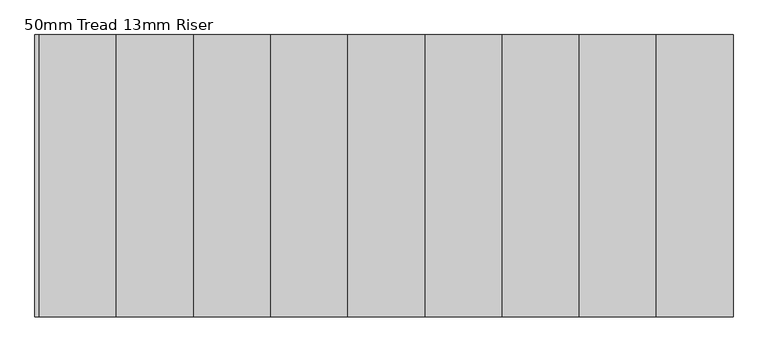
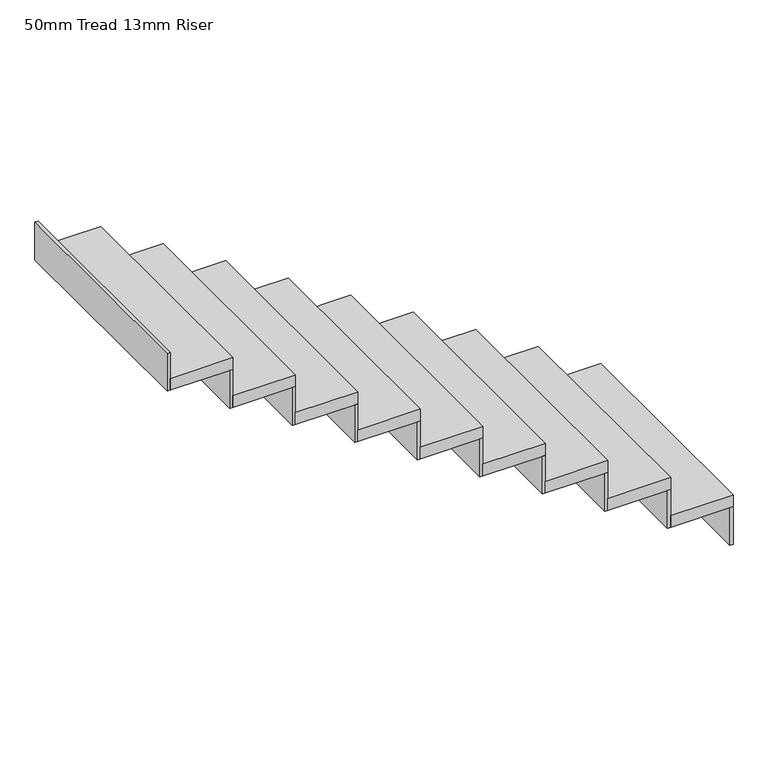
"""IFC4 building model written with IfcOpenShell, lengths in millimetres: stair flight geometry, 50mm Tread 13mm Riser."""

from ifc_helpers import new_model, si_unit, frame, origin, place, context, project, spatial, polyline, outline, extrude, source, transform, mapped, element, save


def stair_flight_50mm_tread_13mm_riser_05b05da2(model_context):
    return source(origin(), model_context, "Body", "SweptSolid", [
        extrude(outline(polyline([(-7557.9329612, -3113.8421603), (-7545.4329612, -3113.8421603), (-7545.4329612, -4028.2421603), (-7557.9329612, -4028.2421603), (-7557.9329612, -3113.8421603)])), frame((0.0, 0.0, 4750.6), z_axis=(0.0, 0.0, 1.0), x_axis=(1.0, 0.0, 0.0)), (0.0, 0.0, 1.0), 160.02),
        extrude(outline(polyline([(-7795.4329612, -4028.2421603), (-7795.4329612, -3113.8421603), (-7545.4329612, -3113.8421603), (-7545.4329612, -4028.2421603), (-7795.4329612, -4028.2421603)])), frame((0.0, 0.0, 4910.62), z_axis=(0.0, 0.0, 1.0), x_axis=(1.0, 0.0, 0.0)), (0.0, 0.0, 1.0), 50.0),
        extrude(outline(polyline([(-7807.9329612, -3113.8421603), (-7795.4329612, -3113.8421603), (-7795.4329612, -4028.2421603), (-7807.9329612, -4028.2421603), (-7807.9329612, -3113.8421603)])), frame((0.0, 0.0, 4910.62), z_axis=(0.0, 0.0, 1.0), x_axis=(1.0, 0.0, 0.0)), (0.0, 0.0, 1.0), 160.02),
        extrude(outline(polyline([(-8045.4329612, -4028.2421603), (-8045.4329612, -3113.8421603), (-7795.4329612, -3113.8421603), (-7795.4329612, -4028.2421603), (-8045.4329612, -4028.2421603)])), frame((0.0, 0.0, 5070.64), z_axis=(0.0, 0.0, 1.0), x_axis=(1.0, 0.0, 0.0)), (0.0, 0.0, 1.0), 50.0),
        extrude(outline(polyline([(-8057.9329612, -3113.8421603), (-8045.4329612, -3113.8421603), (-8045.4329612, -4028.2421603), (-8057.9329612, -4028.2421603), (-8057.9329612, -3113.8421603)])), frame((0.0, 0.0, 5070.64), z_axis=(0.0, 0.0, 1.0), x_axis=(1.0, 0.0, 0.0)), (0.0, 0.0, 1.0), 160.02),
        extrude(outline(polyline([(-8295.4329612, -4028.2421603), (-8295.4329612, -3113.8421603), (-8045.4329612, -3113.8421603), (-8045.4329612, -4028.2421603), (-8295.4329612, -4028.2421603)])), frame((0.0, 0.0, 5230.66), z_axis=(0.0, 0.0, 1.0), x_axis=(1.0, 0.0, 0.0)), (0.0, 0.0, 1.0), 50.0),
        extrude(outline(polyline([(-8307.9329612, -3113.8421603), (-8295.4329612, -3113.8421603), (-8295.4329612, -4028.2421603), (-8307.9329612, -4028.2421603), (-8307.9329612, -3113.8421603)])), frame((0.0, 0.0, 5230.66), z_axis=(0.0, 0.0, 1.0), x_axis=(1.0, 0.0, 0.0)), (0.0, 0.0, 1.0), 160.02),
        extrude(outline(polyline([(-8545.4329612, -4028.2421603), (-8545.4329612, -3113.8421603), (-8295.4329612, -3113.8421603), (-8295.4329612, -4028.2421603), (-8545.4329612, -4028.2421603)])), frame((0.0, 0.0, 5390.68), z_axis=(0.0, 0.0, 1.0), x_axis=(1.0, 0.0, 0.0)), (0.0, 0.0, 1.0), 50.0),
        extrude(outline(polyline([(-8557.9329612, -3113.8421603), (-8545.4329612, -3113.8421603), (-8545.4329612, -4028.2421603), (-8557.9329612, -4028.2421603), (-8557.9329612, -3113.8421603)])), frame((0.0, 0.0, 5390.68), z_axis=(0.0, 0.0, 1.0), x_axis=(1.0, 0.0, 0.0)), (0.0, 0.0, 1.0), 160.02),
        extrude(outline(polyline([(-8795.4329612, -4028.2421603), (-8795.4329612, -3113.8421603), (-8545.4329612, -3113.8421603), (-8545.4329612, -4028.2421603), (-8795.4329612, -4028.2421603)])), frame((0.0, 0.0, 5550.7), z_axis=(0.0, 0.0, 1.0), x_axis=(1.0, 0.0, 0.0)), (0.0, 0.0, 1.0), 50.0),
        extrude(outline(polyline([(-8807.9329612, -3113.8421603), (-8795.4329612, -3113.8421603), (-8795.4329612, -4028.2421603), (-8807.9329612, -4028.2421603), (-8807.9329612, -3113.8421603)])), frame((0.0, 0.0, 5550.7), z_axis=(0.0, 0.0, 1.0), x_axis=(1.0, 0.0, 0.0)), (0.0, 0.0, 1.0), 160.02),
        extrude(outline(polyline([(-9045.4329612, -4028.2421603), (-9045.4329612, -3113.8421603), (-8795.4329612, -3113.8421603), (-8795.4329612, -4028.2421603), (-9045.4329612, -4028.2421603)])), frame((0.0, 0.0, 5710.72), z_axis=(0.0, 0.0, 1.0), x_axis=(1.0, 0.0, 0.0)), (0.0, 0.0, 1.0), 50.0),
        extrude(outline(polyline([(-9057.9329612, -3113.8421603), (-9045.4329612, -3113.8421603), (-9045.4329612, -4028.2421603), (-9057.9329612, -4028.2421603), (-9057.9329612, -3113.8421603)])), frame((0.0, 0.0, 5710.72), z_axis=(0.0, 0.0, 1.0), x_axis=(1.0, 0.0, 0.0)), (0.0, 0.0, 1.0), 160.02),
        extrude(outline(polyline([(-9295.4329612, -4028.2421603), (-9295.4329612, -3113.8421603), (-9045.4329612, -3113.8421603), (-9045.4329612, -4028.2421603), (-9295.4329612, -4028.2421603)])), frame((0.0, 0.0, 5870.74), z_axis=(0.0, 0.0, 1.0), x_axis=(1.0, 0.0, 0.0)), (0.0, 0.0, 1.0), 50.0),
        extrude(outline(polyline([(-9307.9329612, -3113.8421603), (-9295.4329612, -3113.8421603), (-9295.4329612, -4028.2421603), (-9307.9329612, -4028.2421603), (-9307.9329612, -3113.8421603)])), frame((0.0, 0.0, 5870.74), z_axis=(0.0, 0.0, 1.0), x_axis=(1.0, 0.0, 0.0)), (0.0, 0.0, 1.0), 160.02),
        extrude(outline(polyline([(-9545.4329612, -4028.2421603), (-9545.4329612, -3113.8421603), (-9295.4329612, -3113.8421603), (-9295.4329612, -4028.2421603), (-9545.4329612, -4028.2421603)])), frame((0.0, 0.0, 6030.76), z_axis=(0.0, 0.0, 1.0), x_axis=(1.0, 0.0, 0.0)), (0.0, 0.0, 1.0), 50.0),
        extrude(outline(polyline([(-9557.9329612, -3113.8421603), (-9545.4329612, -3113.8421603), (-9545.4329612, -4028.2421603), (-9557.9329612, -4028.2421603), (-9557.9329612, -3113.8421603)])), frame((0.0, 0.0, 6030.76), z_axis=(0.0, 0.0, 1.0), x_axis=(1.0, 0.0, 0.0)), (0.0, 0.0, 1.0), 160.02),
        extrude(outline(polyline([(-9807.9329612, -3113.8421603), (-9795.4329612, -3113.8421603), (-9795.4329612, -4028.2421603), (-9807.9329612, -4028.2421603), (-9807.9329612, -3113.8421603)])), frame((0.0, 0.0, 6190.78), z_axis=(0.0, 0.0, 1.0), x_axis=(1.0, 0.0, 0.0)), (0.0, 0.0, 1.0), 160.02),
        extrude(outline(polyline([(-9795.4329612, -4028.2421603), (-9795.4329612, -3113.8421603), (-9545.4329612, -3113.8421603), (-9545.4329612, -4028.2421603), (-9795.4329612, -4028.2421603)])), frame((0.0, 0.0, 6190.78), z_axis=(0.0, 0.0, 1.0), x_axis=(1.0, 0.0, 0.0)), (0.0, 0.0, 1.0), 50.0),
    ])


if __name__ == "__main__":
    model = new_model("IFC4")
    model_context = context("Model", 3, world=origin())
    ifc_project = project(units=[si_unit("LENGTHUNIT", "METRE", prefix="MILLI")], contexts=[model_context])
    site = spatial("IfcSite", under=ifc_project)
    building = spatial("IfcBuilding", under=site)
    placement = place(None, origin())
    stair_flight_50mm_tread_13mm_riser_shape = stair_flight_50mm_tread_13mm_riser_05b05da2(model_context)
    element("IfcStairFlight", 1, ObjectType="50mm Tread 13mm Riser", at=placement, inside=building, context=model_context, shape_type="MappedRepresentation", body=[
        mapped(stair_flight_50mm_tread_13mm_riser_shape, transform((0.0, 0.0, 0.0), x_axis=(1.0, 0.0, 0.0), y_axis=(0.0, 1.0, 0.0), z_axis=(0.0, 0.0, 1.0))),
    ])
    save(model, "model.ifc")
